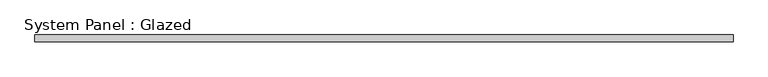
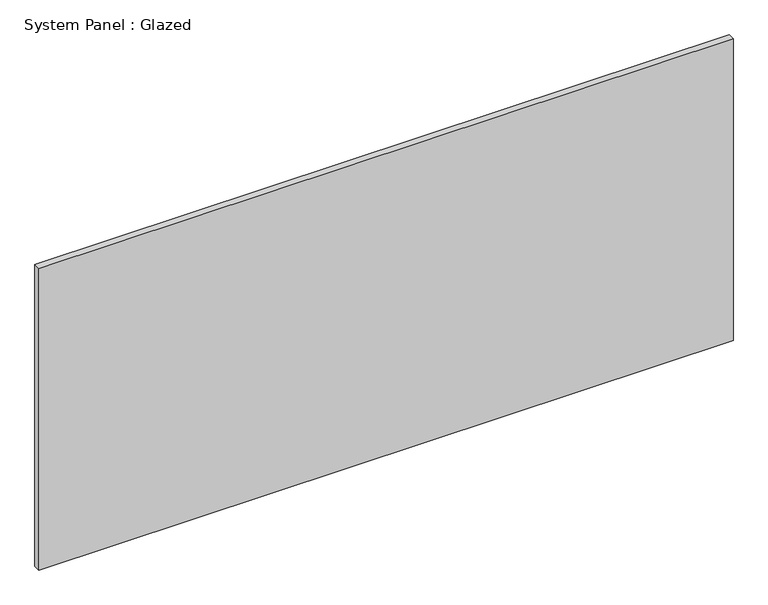
"""IFC4 building model written with IfcOpenShell, lengths in millimetres: plate geometry, System Panel : Glazed."""

from ifc_helpers import new_model, si_unit, origin, origin_with_axes, place, context, project, spatial, polyline, outline, extrude, source, transform, mapped, element, save


def system_panel_glazed_b99798ed(model_context):
    return source(origin(), model_context, "Body", "SweptSolid", [
        extrude(outline(polyline([(1326.373489, 19.05), (-1326.373489, 19.05), (-1326.373489, 44.45), (1326.373489, 44.45), (1326.373489, 19.05)])), origin_with_axes(), (0.0, 0.0, 1.0), 1219.2),
    ])


if __name__ == "__main__":
    model = new_model("IFC4")
    model_context = context("Model", 3, world=origin())
    ifc_project = project(units=[si_unit("LENGTHUNIT", "METRE", prefix="MILLI")], contexts=[model_context])
    site = spatial("IfcSite", under=ifc_project)
    building = spatial("IfcBuilding", under=site)
    placement = place(None, origin())
    system_panel_glazed_shape = system_panel_glazed_b99798ed(model_context)
    element("IfcPlate", 1, ObjectType="System Panel : Glazed", at=placement, inside=building, context=model_context, shape_type="MappedRepresentation", body=[
        mapped(system_panel_glazed_shape, transform((0.0, 0.0, 0.0), x_axis=(1.0, 0.0, 0.0), y_axis=(0.0, 1.0, 0.0), z_axis=(0.0, 0.0, 1.0))),
    ])
    save(model, "model.ifc")

# Revit data of these elements
# Type "System Panel : Glazed"
#   Construction Type Id = "GSP4R"
#   Analytic Construction = "1/8 in Pilkington single glazing"
#   Visual Light Transmittance = 0.9
#   Solar Heat Gain Coefficient = 0.86
#   Heat Transfer Coefficient (U) = 1.18115 BTU/(h·ft²·°F)
# Element 1 (IfcPlate, "System Panel : Glazed")
#   Materials on its faces: "Glass"
# Materials
#   "Glass": class "Glass", colour RGB 0 128 192, transparency 0.75, Description = "Soda Lime Glass", Cost = 0
